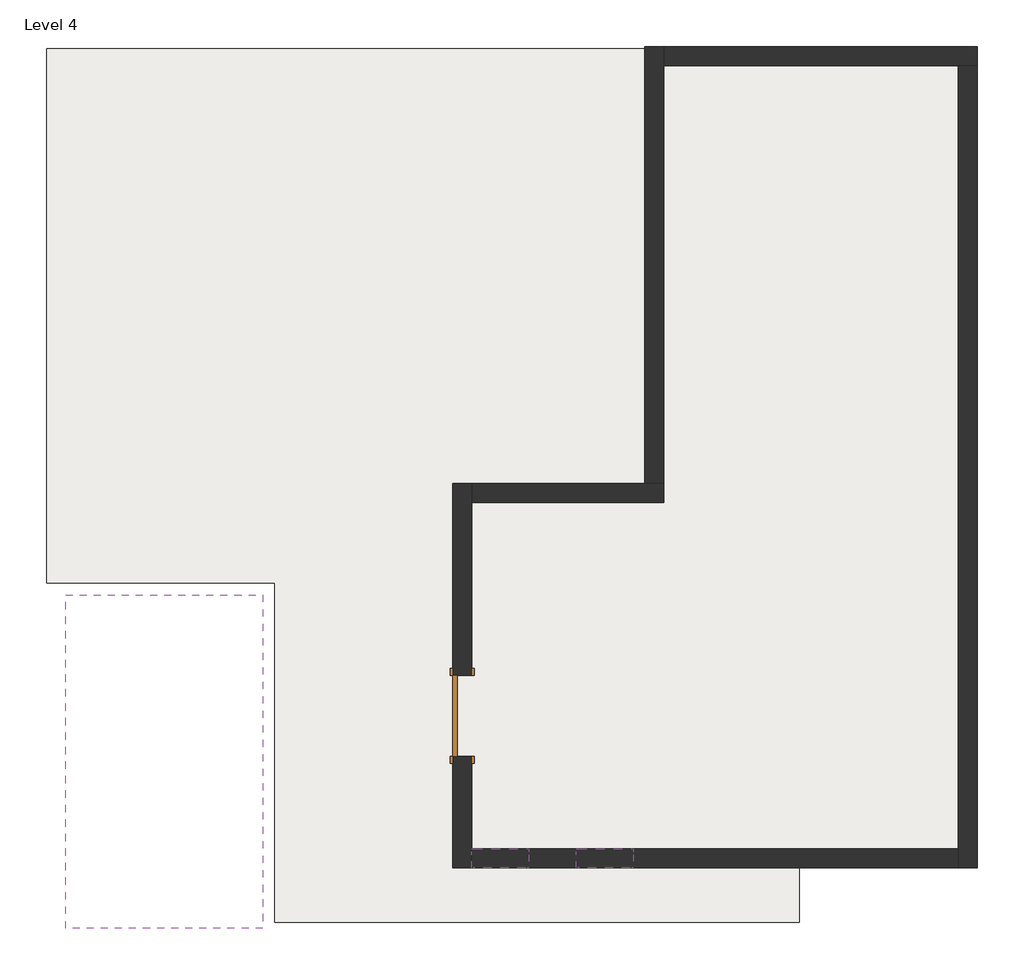
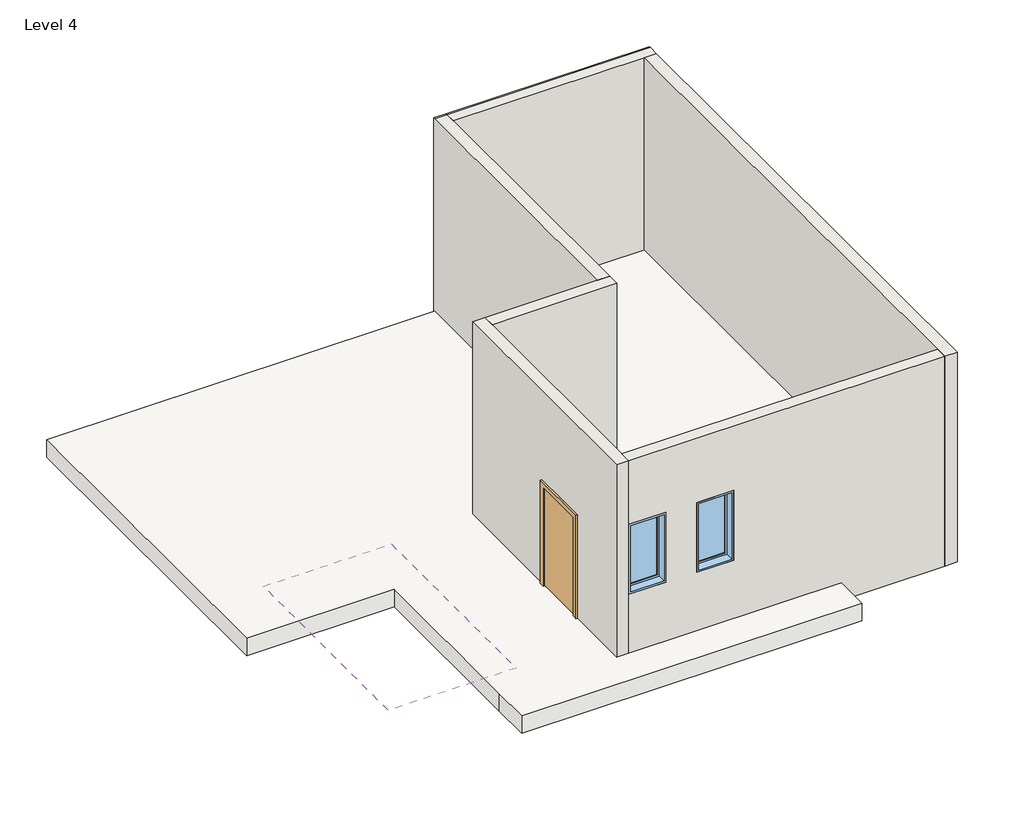
# One storey: 6 walls, 2 roofs, 2 windows, 1 door.
"""IFC4 building model written with IfcOpenShell, lengths in millimetres."""

from ifc_helpers import new_model, si_unit, frame, origin, place, context, project, spatial, polyline, outline, extrude, faceted_brep, transform, mapped, element, save
from components import door_10fd3a06, window_80bd9af0

model = new_model("IFC4")

# Units and contexts
model_context = context("Model", 3, world=origin())
ifc_project = project(units=[si_unit("LENGTHUNIT", "METRE", prefix="MILLI")], contexts=[model_context])

# Site, building, storey
site = spatial("IfcSite", under=ifc_project)
building = spatial("IfcBuilding", under=site)
storey = spatial("IfcBuildingStorey", under=building, Name="Level 4", Elevation=10972.8)

# Door
placement = place(None, origin())
door_shape = door_10fd3a06(model_context)
element("IfcDoor", 1, ObjectType="Door-Single-Panel : 34\" x 80\"", at=placement, inside=storey, context=model_context, shape_type="MappedRepresentation", body=[
    mapped(door_shape, transform((-7854.7432037, 2872.8548743, 10972.8), x_axis=(0.0, 1.0, 0.0), y_axis=(-1.0, 0.0, 0.0), z_axis=(0.0, 0.0, 1.0))),
])

# Roofs
element("IfcRoof", 2, ObjectType="Generic - 12\"", at=placement, inside=storey, context=model_context, shape_type="SweptSolid", body=[
    extrude(outline(polyline([(-12299.7432037, 10010.2548743), (-2342.9432037, 10010.2548743), (-2342.9432037, 1247.2548743), (-4247.9432037, 1247.2548743), (-4247.9432037, 663.0548743), (-9861.3432037, 663.0548743), (-9861.3432037, 1298.0548743), (-9861.3432037, 4295.2548743), (-12299.7432037, 4295.2548743), (-12299.7432037, 10010.2548743)])), frame((0.0, 0.0, 10972.8), z_axis=(0.0, 0.0, 1.0), x_axis=(1.0, 0.0, 0.0)), (0.0, 0.0, 1.0), 304.8),
])
element("IfcRoof", 3, ObjectType="Generic - 12\"", at=placement, inside=storey, context=model_context, shape_type="SweptSolid", body=[
    extrude(outline(polyline([(-12096.5432037, 4168.2548743), (-9988.3432037, 4168.2548743), (-9988.3432037, 599.5548476), (-12096.5432037, 599.5548476), (-12096.5432037, 4168.2548743)])), frame((0.0, 0.0, 12192.0), z_axis=(0.0, 0.0, 1.0), x_axis=(1.0, 0.0, 0.0)), (0.0, 0.0, 1.0), 304.8),
])

# Walls
element("IfcWall", 4, ObjectType="Generic - 8\"", at=placement, inside=storey, context=model_context, shape_type="Brep", body=[
    faceted_brep([(-7753.1432037, 3304.6548743, 13004.8), (-7753.1432037, 3304.6548743, 10972.8), (-7753.1432037, 5158.8548743, 10972.8), (-7753.1432037, 5362.0548743, 10972.8), (-7753.1432037, 5362.0548743, 14630.4), (-7753.1432037, 5158.8548743, 14630.4), (-7753.1432037, 1450.4548743, 14630.4), (-7753.1432037, 1247.2548743, 14630.4), (-7753.1432037, 1247.2548743, 13520.2862521), (-7753.1432037, 1247.2548743, 12301.0862521), (-7753.1432037, 1247.2548743, 10972.8), (-7753.1432037, 1450.4548743, 10972.8), (-7753.1432037, 2441.0548743, 10972.8), (-7753.1432037, 2441.0548743, 13004.8), (-7956.3432037, 5362.0548743, 10972.8), (-7956.3432037, 3304.6548743, 10972.8), (-7956.3432037, 3304.6548743, 13004.8), (-7956.3432037, 2441.0548743, 13004.8), (-7956.3432037, 2441.0548743, 10972.8), (-7956.3432037, 1247.2548743, 10972.8), (-7956.3432037, 1247.2548743, 14630.4), (-7956.3432037, 5362.0548743, 14630.4)], [[[0, 1, 2, 3, 4, 5, 6, 7, 8, 9, 10, 11, 12, 13]], [[14, 15, 16, 17, 18, 19, 20, 21]], [[12, 11, 10, 19, 18]], [[3, 2, 1, 15, 14]], [[4, 3, 14, 21]], [[10, 9, 8, 7, 20, 19]], [[7, 6, 5, 4, 21, 20]], [[16, 15, 1, 0]], [[17, 16, 0, 13]], [[18, 17, 13, 12]]]),
])
element("IfcWall", 5, ObjectType="Generic - 8\"", at=placement, inside=storey, context=model_context, shape_type="Brep", body=[
    faceted_brep([(-7753.1432037, 5158.8548743, 10972.8), (-5695.7432037, 5158.8548743, 10972.8), (-5695.7432037, 5158.8548743, 14630.4), (-7753.1432037, 5158.8548743, 14630.4), (-7753.1432037, 5362.0548743, 10972.8), (-7753.1432037, 5362.0548743, 14630.4), (-5898.9432037, 5362.0548743, 14630.4), (-5695.7432037, 5362.0548743, 14630.4), (-5695.7432037, 5362.0548743, 10972.8), (-5898.9432037, 5362.0548743, 10972.8)], [[[0, 1, 2, 3]], [[4, 5, 6, 7, 8, 9]], [[1, 0, 4, 9, 8]], [[0, 3, 5, 4]], [[2, 1, 8, 7]], [[3, 2, 7, 6, 5]]]),
])
element("IfcWall", 6, ObjectType="Generic - 8\"", at=placement, inside=storey, context=model_context, shape_type="Brep", body=[
    faceted_brep([(-5695.7432037, 5362.0548743, 10972.8), (-5695.7432037, 9832.4548743, 10972.8), (-5695.7432037, 10010.2548743, 10972.8), (-5695.7432037, 10035.6548743, 10972.8), (-5695.7432037, 10035.6548743, 14630.4), (-5695.7432037, 10010.2548743, 14630.4), (-5695.7432037, 9832.4548743, 14630.4), (-5695.7432037, 5362.0548743, 14630.4), (-5898.9432037, 5362.0548743, 10972.8), (-5898.9432037, 5362.0548743, 14630.4), (-5898.9432037, 10010.2548743, 14630.4), (-5898.9432037, 10035.6548743, 14630.4), (-5898.9432037, 10035.6548743, 10972.8), (-5898.9432037, 10010.2548743, 10972.8)], [[[0, 1, 2, 3, 4, 5, 6, 7]], [[8, 9, 10, 11, 12, 13]], [[3, 2, 1, 0, 8, 13, 12]], [[0, 7, 9, 8]], [[5, 4, 11, 10]], [[7, 6, 5, 10, 9]], [[3, 12, 11, 4]]]),
])
element("IfcWall", 7, ObjectType="Generic - 8\"", at=placement, inside=storey, context=model_context, shape_type="Brep", body=[
    faceted_brep([(-5695.7432037, 9832.4548743, 14630.4), (-5695.7432037, 9832.4548743, 10972.8), (-2546.1432037, 9832.4548743, 10972.8), (-2342.9432037, 9832.4548743, 10972.8), (-2342.9432037, 9832.4548743, 14630.4), (-2546.1432037, 9832.4548743, 14630.4), (-5695.7432037, 10035.6548743, 10972.8), (-5695.7432037, 10035.6548743, 14630.4), (-2342.9432037, 10035.6548743, 14630.4), (-2342.9432037, 10035.6548743, 10972.8), (-5695.7432037, 10010.2548743, 10972.8), (-2342.9432037, 10010.2548743, 14630.4), (-5695.7432037, 10010.2548743, 14630.4)], [[[0, 1, 2, 3, 4, 5]], [[6, 7, 8, 9]], [[3, 2, 1, 10, 6, 9]], [[4, 3, 9, 8, 11]], [[11, 8, 7, 12]], [[0, 5, 4, 11, 12]], [[0, 12, 7, 6, 10, 1]]]),
])
element("IfcWall", 8, ObjectType="Generic - 8\"", at=placement, inside=storey, context=model_context, shape_type="Brep", body=[
    faceted_brep([(-2546.1432037, 9832.4548743, 10972.8), (-2546.1432037, 1450.4548743, 10972.8), (-2546.1432037, 1247.2548743, 10972.8), (-2546.1432037, 1247.2548743, 14630.4), (-2546.1432037, 1450.4548743, 14630.4), (-2546.1432037, 9832.4548743, 14630.4), (-2342.9432037, 9832.4548743, 10972.8), (-2342.9432037, 9832.4548743, 14630.4), (-2342.9432037, 1247.2548743, 14630.4), (-2342.9432037, 1247.2548743, 10972.8)], [[[0, 1, 2, 3, 4, 5]], [[6, 7, 8, 9]], [[2, 1, 0, 6, 9]], [[0, 5, 7, 6]], [[3, 2, 9, 8]], [[5, 4, 3, 8, 7]]]),
])
element("IfcWall", 9, ObjectType="Generic - 8\"", at=placement, inside=storey, context=model_context, shape_type="SweptSolid", body=[
    extrude(outline(polyline([(10972.8, -7753.1432037), (10972.8, -2546.1432037), (14630.4, -2546.1432037), (14630.4, -7753.1432037), (13520.2862521, -7753.1432037), (13520.2862521, -7143.5432037), (12301.0862521, -7143.5432037), (12301.0862521, -7753.1432037), (10972.8, -7753.1432037)]), holes=[polyline([(13511.1892623, -6025.9432037), (12291.9892623, -6025.9432037), (12291.9892623, -6635.5432037), (13511.1892623, -6635.5432037), (13511.1892623, -6025.9432037)])]), frame((0.0, 1247.2548743, 0.0), z_axis=(0.0, 1.0, 0.0), x_axis=(0.0, 0.0, 1.0)), (0.0, 0.0, 1.0), 203.2),
])

# Windows
window_shape = window_80bd9af0(model_context)
element("IfcWindow", 10, ObjectType="Fixed : 24\" x 48\"", at=placement, inside=storey, context=model_context, shape_type="MappedRepresentation", body=[
    mapped(window_shape, transform((-7410.2432037, 1348.8548743, 11386.6862521), x_axis=(1.0, 0.0, 0.0), y_axis=(0.0, 1.0, 0.0), z_axis=(0.0, 0.0, 1.0))),
])
element("IfcWindow", 11, ObjectType="Fixed : 24\" x 48\"", at=placement, inside=storey, context=model_context, shape_type="MappedRepresentation", body=[
    mapped(window_shape, transform((-6292.6432037, 1348.8548743, 11377.5892623), x_axis=(1.0, 0.0, 0.0), y_axis=(0.0, 1.0, 0.0), z_axis=(0.0, 0.0, 1.0))),
])

save(model, "model.ifc")

# Revit data of these elements
# Type "Door-Single-Panel : 34\" x 80\""
#   Type Mark = "9"
#   Construction Type Id = "DOOR"
#   Assembly Code = "C1020300"
#   Analytic Construction = "Wooden"
#   Thickness = 0' - 2"
#   Thermal Resistance (R) = 2.5876 (h·ft²·°F)/BTU
#   Swing Angle [instance default] = 90.00°
#   Heat Transfer Coefficient (U) = 0.3865 BTU/(h·ft²·°F)
#   Height = 6' - 8"
#   Trim Projection Ext = 0' - 1"
#   Trim Projection Int = 0' - 1"
#   Trim Width = 0' - 3"
#   Width = 2' - 10"
#   Define Thermal Properties by = 1
#   Panel Material = Wood - Birch - Solid Stained Light Low Gloss
#   Trim Material = Paint - Sienna
#   Visual Light Transmittance = 0
#   Solar Heat Gain Coefficient = 0
#   Function = (empty or 0)
#   Wall Closure = (empty or 0)
# Type "Generic - 12\""
#   Assembly Code = "B1020"
#   Layers, outside or top first: 1' - 0" no material (function 1)
# Type "Generic - 8\""
#   Assembly Code = "B2010"
#   Layers, outside or top first: 0' - 8" no material (function 1)
# Type "Fixed : 24\" x 48\""
#   Type Mark = "2"
#   Construction Type Id = "GSP4R"
#   Assembly Code = "B2020100"
#   Analytic Construction = "1/8 in Pilkington single glazing"
#   Visual Light Transmittance = 0.9
#   Solar Heat Gain Coefficient = 0.78
#   Heat Transfer Coefficient (U) = 0.6496 BTU/(h·ft²·°F)
#   Height = 4' - 0"
#   Default Sill Height = 3' - 0"
#   Width = 2' - 0"
#   Window Inset = 0' - 0 3/4"
#   Define Thermal Properties by = 1
#   Glass Pane Material = Glass
#   Sash Material = Sash
#   Wall Closure = (empty or 0)
# Element 1 (IfcDoor, "Door-Single-Panel : 34\" x 80\"")
#   Swing Angle = 90.00°
#   Phase Created = New Construction
#   Materials on its faces: "Paint - Sienna", "Wood - Birch - Solid Stained Light Low Gloss"
# Element 2 (IfcRoof, "Generic - 12\"")
#   built-in parameter 1001705 = 37 (stored number, unit not read)
#   built-in parameter 1001710 = 33615
#   Phase Created = New Construction
#   Materials on its faces: "Default Roof"
# Element 3 (IfcRoof, "Generic - 12\"")
#   built-in parameter 1001705 = 41 (stored number, unit not read)
#   built-in parameter 1001701 = 4 (stored number, unit not read)
#   built-in parameter 1001710 = 33615
#   Phase Created = New Construction
#   Materials on its faces: "Default Roof"
# Elements 4, 5, 6, 7, 8, 9 (IfcWall, "Generic - 8\"")
#   Top Offset = 0' - 0"
#   Base Offset = 0' - 0"
#   Unconnected Height = 12' - 0"
#   wall height = 12' - 0"
#   Phase Created = New Construction
#   Base Constraint = Level 4
#   Materials on its faces: "Default Wall"
# Element 10 (IfcWindow, "Fixed : 24\" x 48\"")
#   Mark = "3"
#   Phase Created = New Construction
#   Materials on its faces: "Sash", "Glass"
# Element 11 (IfcWindow, "Fixed : 24\" x 48\"")
#   Mark = "4"
#   Phase Created = New Construction
#   Materials on its faces: "Sash", "Glass"
# Materials
#   "Wood - Birch - Solid Stained Light Low Gloss": class "Wood", colour RGB 210 159 95, transparency 0, Cost = 0
#   "Paint - Sienna": colour RGB 118 70 51, transparency 0, Cost = 0
#   "Glass": class "Glass", colour RGB 0 128 192, transparency 0.75, Description = "Soda Lime Glass", Cost = 0
#   "Sash": class "Wood", colour RGB 224 178 126, transparency 0
#   "Default Roof": colour RGB 88 101 114, transparency 0
#   "Default Wall": colour RGB 128 128 128, transparency 0
